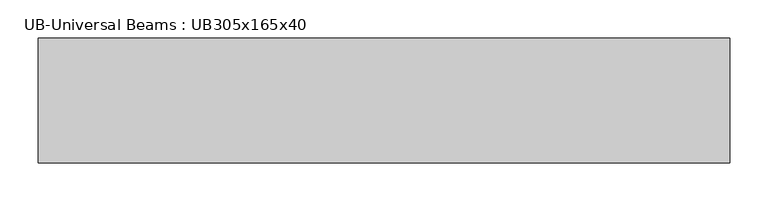
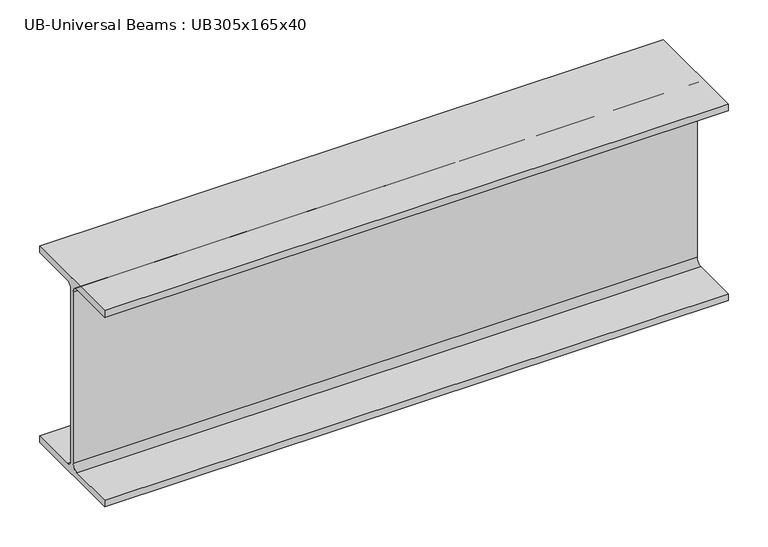
"""IFC4 building model written with IfcOpenShell, lengths in millimetres: beam geometry, UB-Universal Beams : UB305x165x40."""

from ifc_helpers import new_model, si_unit, point, frame, frame_2d, origin, place, context, project, spatial, polyline, circle_curve, trimmed, segment, composite_curve, outline, extrude, source, transform, mapped, element, save


def ub_universal_beams_ub305x165x40_0b90c1cb(model_context):
    return source(origin(), model_context, "Body", "SweptSolid", [
        extrude(outline(composite_curve([segment(polyline([(82.5, -141.5), (82.5, -151.7), (-82.5, -151.7), (-82.5, -141.5), (-11.9, -141.5)]), True, "CONTINUOUS"), segment(trimmed(circle_curve(frame_2d((-11.9, -132.6)), 8.9), [point((-11.9, -141.5))], [point((-3.0, -132.6))], True, "CARTESIAN"), True, "CONTINUOUS"), segment(polyline([(-3.0, -132.6), (-3.0, 132.6)]), True, "CONTINUOUS"), segment(trimmed(circle_curve(frame_2d((-11.9, 132.6)), 8.9), [point((-3.0, 132.6))], [point((-11.9, 141.5))], True, "CARTESIAN"), True, "CONTINUOUS"), segment(polyline([(-11.9, 141.5), (-82.5, 141.5), (-82.5, 151.7), (82.5, 151.7), (82.5, 141.5), (11.9, 141.5)]), True, "CONTINUOUS"), segment(trimmed(circle_curve(frame_2d((11.9, 132.6)), 8.9), [point((11.9, 141.5))], [point((3.0, 132.6))], True, "CARTESIAN"), True, "CONTINUOUS"), segment(polyline([(3.0, 132.6), (3.0, -132.6)]), True, "CONTINUOUS"), segment(trimmed(circle_curve(frame_2d((11.9, -132.6)), 8.9), [point((3.0, -132.6))], [point((11.9, -141.5))], True, "CARTESIAN"), True, "CONTINUOUS"), segment(polyline([(11.9, -141.5), (82.5, -141.5)]), True, "CONTINUOUS")], self_intersect=False)), frame((-1086.3, 0.0, 0.0), z_axis=(1.0, 0.0, 0.0), x_axis=(0.0, 1.0, 0.0)), (0.0, 0.0, 1.0), 910.4),
    ])


if __name__ == "__main__":
    model = new_model("IFC4")
    model_context = context("Model", 3, world=origin())
    ifc_project = project(units=[si_unit("LENGTHUNIT", "METRE", prefix="MILLI")], contexts=[model_context])
    site = spatial("IfcSite", under=ifc_project)
    building = spatial("IfcBuilding", under=site)
    placement = place(None, origin())
    ub_universal_beams_ub305x165x40_shape = ub_universal_beams_ub305x165x40_0b90c1cb(model_context)
    element("IfcBeam", 1, ObjectType="UB-Universal Beams : UB305x165x40", at=placement, inside=building, context=model_context, shape_type="MappedRepresentation", body=[
        mapped(ub_universal_beams_ub305x165x40_shape, transform((0.0, 0.0, 0.0), x_axis=(1.0, 0.0, 0.0), y_axis=(0.0, 1.0, 0.0), z_axis=(0.0, 0.0, 1.0))),
    ])
    save(model, "model.ifc")

# Revit data of these elements
# Type "UB-Universal Beams : UB305x165x40"
#   Section Name Key = "UB305X165X40"
#   Width = 16.5 cm
#   Web Thickness = 0.6 cm
#   Web Fillet = 0.89 cm
#   Warping Constant = 164000.0 cm⁶
#   Torsional Moment of Inertia = 14.70 cm⁴
#   Section Area = 51.3 cm²
#   Plastic Modulus weak axis = 142.0 cm³
#   Plastic Modulus strong axis = 623.0 cm³
#   Nominal Weight = 40.2999 kgf/m
#   Moment of Inertia weak axis = 764.00 cm⁴
#   Moment of Inertia strong axis = 8503.00 cm⁴
#   Height = 30.34 cm
#   Flange Thickness = 1.02 cm
#   Elastic Modulus weak axis = 92.6 cm³
#   Elastic Modulus strong axis = 560.0 cm³
#   Centroid Vertical = 15.17 cm
#   Centroid Horizontal = 8.25 cm
#   Bolt Spacing = 9.0 cm
#   Length [instance default] = 1500 mm
#   Structural Material [instance default] = Metal - Steel 43-275
#   Type Comments = ""
#   Assembly Code = ""
# Element 1 (IfcBeam, "UB-Universal Beams : UB305x165x40")
#   Materials on its faces: "Metal - Steel 43-275"
# Materials
#   "Metal - Steel 43-275": class "Metal", colour RGB 247 247 247, transparency 0, Cost = 0
